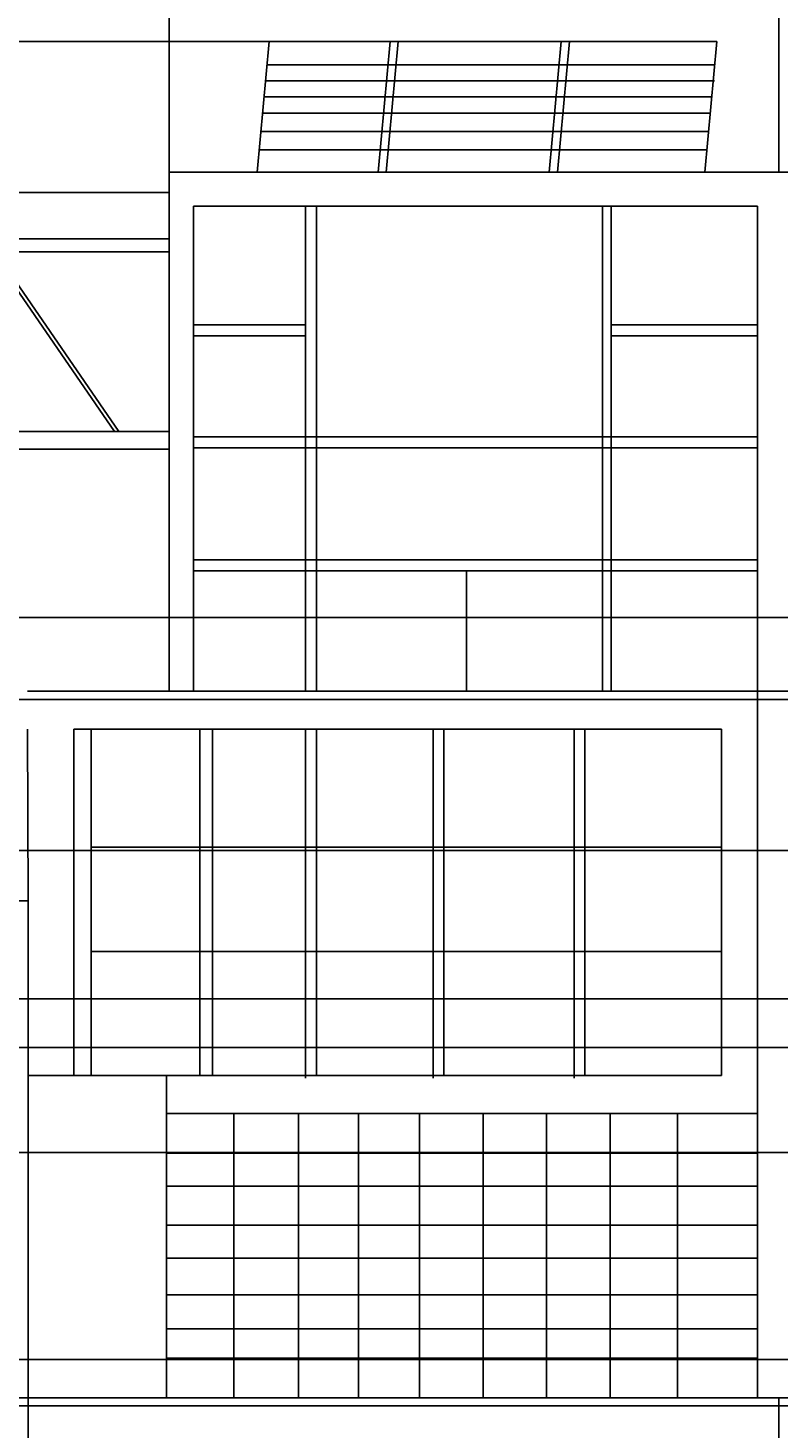
# Model space of a CAD drawing. Units: inches. Extents: x -32109 to 33221, y -19197 to 7608.
# Tile 5 of 25: x -6953 to -4279, y -16323 to -11338. Entities that reach past the tile are written whole.
import ezdxf

# ---------------------------------------------------------------- set-up
doc = ezdxf.new("R2010")
doc.units = ezdxf.units.IN
doc.header["$MEASUREMENT"] = 0
doc.layers.add('A-ANNO-DIMS', color=2, linetype='Continuous', lineweight=18)
doc.layers.add('A-ELEV', color=7, linetype='Continuous', lineweight=25)
doc.styles.get("Standard").update_dxf_attribs({"font": 'arial.ttf'})
doc.dimstyles.get("Standard").update_dxf_attribs({"dimtxt": 0.18, "dimasz": 0.18, "dimexe": 0.18, "dimexo": 0.0625, "dimgap": 0.09, "dimtad": 0, "dimtih": 1, "dimtoh": 1, "dimdec": 4, "dimzin": 0, "dimdsep": 46, "dimtxsty": 'Standard', "dimcen": 0.09, "dimadec": 0, "dimazin": 0, "dimtfac": 1, "dimtdec": 4, "dimtofl": 0, "dimtmove": 0, "dimatfit": 3, "dimfxl": 1, "dimtolj": 1, "dimtzin": 0, "dimarcsym": 0})

# ---------------------------------------------------------------- blocks, each defined once
blk = doc.blocks.new('*D13')
at = {"layer": 'A-ANNO-DIMS', "color": 0, "lineweight": -2, "transparency": 16777216}
for p, q in [((-21916.3, -16214.9), (-21916.3, -19197.3)), ((5067.2, -16244.2), (5067.2, -19197.3)), ((-21916.1, -19197.2), (-8425, -19197.2)), ((5067, -19197.2), (-8424.2, -19197.2))]:
    blk.add_line(p, q, dxfattribs=at)
at = {"layer": 'A-ANNO-DIMS', "color": 0, "transparency": 16777216}
for points in [[(-21916.1, -19197.1), (-21916.1, -19197.2), (-21916.3, -19197.2)], [(5067, -19197.1), (5067, -19197.2), (5067.2, -19197.2)]]:
    blk.add_solid(points, dxfattribs=at)
at = {"layer": 'Defpoints', "color": 0, "transparency": 16777216}
for p in [(-21916.3, -16214.8), (5067.2, -16244.1), (5067.2, -19197.2)]:
    blk.add_point(p, dxfattribs=at)
at = {"layer": 'A-ANNO-DIMS', "color": 0, "transparency": 16777216, "insert": (-8424.6, -19197.2), "char_height": 0.18, "attachment_point": 5}
blk.add_mtext('\\A1;26983', dxfattribs=at)
blk = doc.blocks.new('*D14')
at = {"layer": 'A-ANNO-DIMS', "color": 0, "lineweight": -2, "transparency": 16777216}
for p, q in [((-18893.9, -10978.7), (-32108.4, -10978.7)), ((-32108.2, -10978.9), (-32108.2, -13611.2)), ((-32108.2, -16243.9), (-32108.2, -13611.6)), ((5067.1, -16244.1), (-32108.4, -16244.1))]:
    blk.add_line(p, q, dxfattribs=at)
at = {"layer": 'A-ANNO-DIMS', "color": 0, "transparency": 16777216}
for points in [[(-32108.2, -10978.9), (-32108.2, -10978.9), (-32108.2, -10978.7)], [(-32108.2, -16243.9), (-32108.2, -16243.9), (-32108.2, -16244.1)]]:
    blk.add_solid(points, dxfattribs=at)
at = {"layer": 'Defpoints', "color": 0, "transparency": 16777216}
for p in [(-18893.8, -10978.7), (-32108.2, -16244.1), (5067.2, -16244.1)]:
    blk.add_point(p, dxfattribs=at)
at = {"layer": 'A-ANNO-DIMS', "color": 0, "transparency": 16777216, "insert": (-32108.2, -13611.4), "char_height": 0.18, "attachment_point": 5}
blk.add_mtext('\\A1;5265', dxfattribs=at)
blk = doc.blocks.new('*D15')
at = {"layer": 'A-ANNO-DIMS', "color": 0, "lineweight": -2, "transparency": 16777216}
for p, q in [((-8664.1, -16214.9), (-8664.1, -19197.3)), ((-6952.8, -16214.9), (-6952.8, -19197.3)), ((-8664, -19197.2), (-7808.9, -19197.2)), ((-6953, -19197.2), (-7808, -19197.2))]:
    blk.add_line(p, q, dxfattribs=at)
at = {"layer": 'A-ANNO-DIMS', "color": 0, "transparency": 16777216}
for points in [[(-8664, -19197.1), (-8664, -19197.2), (-8664.1, -19197.2)], [(-6953, -19197.1), (-6953, -19197.2), (-6952.8, -19197.2)]]:
    blk.add_solid(points, dxfattribs=at)
at = {"layer": 'Defpoints', "color": 0, "transparency": 16777216}
for p in [(-8664.1, -16214.8), (-6952.8, -16214.8), (-6952.8, -19197.2)]:
    blk.add_point(p, dxfattribs=at)
at = {"layer": 'A-ANNO-DIMS', "color": 0, "transparency": 16777216, "insert": (-7808.5, -19197.2), "char_height": 0.18, "attachment_point": 5}
blk.add_mtext('\\A1;1711.4', dxfattribs=at)
blk = doc.blocks.new('*D23')
at = {"layer": 'A-ANNO-DIMS', "color": 0, "lineweight": -2, "transparency": 16777216}
for p, q in [((-4093.7, -14968.1), (-32108.4, -14968.1)), ((-32108.2, -14968.3), (-32108.2, -15591.3)), ((-32108.2, -16214.6), (-32108.2, -15591.6)), ((-4279, -16214.8), (-32108.4, -16214.8))]:
    blk.add_line(p, q, dxfattribs=at)
at = {"layer": 'A-ANNO-DIMS', "color": 0, "transparency": 16777216}
for points in [[(-32108.2, -14968.3), (-32108.2, -14968.3), (-32108.2, -14968.1)], [(-32108.2, -16214.6), (-32108.2, -16214.6), (-32108.2, -16214.8)]]:
    blk.add_solid(points, dxfattribs=at)
at = {"layer": 'Defpoints', "color": 0, "transparency": 16777216}
for p in [(-32108.2, -14968.1), (-4093.7, -14968.1), (-4279, -16214.8)]:
    blk.add_point(p, dxfattribs=at)
at = {"layer": 'A-ANNO-DIMS', "color": 0, "transparency": 16777216, "insert": (-32108.2, -15591.4), "char_height": 0.18, "attachment_point": 5}
blk.add_mtext('\\A1;1246.7', dxfattribs=at)
blk = doc.blocks.new('*D88')
at = {"layer": 'A-ANNO-DIMS', "color": 0, "lineweight": -2, "transparency": 16777216}
for p, q in [((-6450, -11924), (-32108.4, -11924)), ((-32108.2, -11924.1), (-32108.2, -12380.7)), ((-32108.2, -12837.6), (-32108.2, -12381)), ((-6450, -12837.7), (-32108.4, -12837.7))]:
    blk.add_line(p, q, dxfattribs=at)
at = {"layer": 'A-ANNO-DIMS', "color": 0, "transparency": 16777216}
for points in [[(-32108.2, -11924.1), (-32108.2, -11924.1), (-32108.2, -11924)], [(-32108.2, -12837.6), (-32108.2, -12837.6), (-32108.2, -12837.7)]]:
    blk.add_solid(points, dxfattribs=at)
at = {"layer": 'Defpoints', "color": 0, "transparency": 16777216}
for p in [(-6450, -11924), (-32108.2, -12837.7), (-6450, -12837.7)]:
    blk.add_point(p, dxfattribs=at)
at = {"layer": 'A-ANNO-DIMS', "color": 0, "transparency": 16777216, "insert": (-32108.2, -12380.9), "char_height": 0.18, "attachment_point": 5}
blk.add_mtext('\\A1;913.8', dxfattribs=at)
blk = doc.blocks.new('*D92')
at = {"layer": 'A-ANNO-DIMS', "color": 0, "lineweight": -2, "transparency": 16777216}
for p, q in [((-8664.1, -13437.2), (9252.7, -13437.2)), ((9252.5, -13437.4), (9252.5, -14825.8)), ((9252.5, -16214.6), (9252.5, -14826.2)), ((-8664.1, -16214.8), (9252.7, -16214.8))]:
    blk.add_line(p, q, dxfattribs=at)
at = {"layer": 'A-ANNO-DIMS', "color": 0, "transparency": 16777216}
for points in [[(9252.5, -13437.4), (9252.5, -13437.4), (9252.5, -13437.2)], [(9252.5, -16214.6), (9252.5, -16214.6), (9252.5, -16214.8)]]:
    blk.add_solid(points, dxfattribs=at)
at = {"layer": 'Defpoints', "color": 0, "transparency": 16777216}
for p in [(-8664.1, -13437.2), (-8664.1, -16214.8), (9252.5, -16214.8)]:
    blk.add_point(p, dxfattribs=at)
at = {"layer": 'A-ANNO-DIMS', "color": 0, "transparency": 16777216, "insert": (9252.5, -14826), "char_height": 0.18, "attachment_point": 5}
blk.add_mtext('\\A1;2777.6', dxfattribs=at)
blk = doc.blocks.new('*D99')
at = {"layer": 'A-ANNO-DIMS', "color": 0, "lineweight": -2, "transparency": 16777216}
for p, q in [((-9175.1, -13729), (9252.7, -13729)), ((9252.5, -13729.2), (9252.5, -13997.5)), ((9252.5, -14266.2), (9252.5, -13997.9)), ((-9175.1, -14266.4), (9252.7, -14266.4))]:
    blk.add_line(p, q, dxfattribs=at)
at = {"layer": 'A-ANNO-DIMS', "color": 0, "transparency": 16777216}
for points in [[(9252.5, -13729.2), (9252.5, -13729.2), (9252.5, -13729)], [(9252.5, -14266.2), (9252.5, -14266.2), (9252.5, -14266.4)]]:
    blk.add_solid(points, dxfattribs=at)
at = {"layer": 'Defpoints', "color": 0, "transparency": 16777216}
for p in [(-9175.2, -13729), (-9175.2, -14266.4), (9252.5, -14266.4)]:
    blk.add_point(p, dxfattribs=at)
at = {"layer": 'A-ANNO-DIMS', "color": 0, "transparency": 16777216, "insert": (9252.5, -13997.7), "char_height": 0.18, "attachment_point": 5}
blk.add_mtext('\\A1;537.4', dxfattribs=at)
blk = doc.blocks.new('*D100')
at = {"layer": 'A-ANNO-DIMS', "color": 0, "lineweight": -2, "transparency": 16777216}
for p, q in [((-9175.1, -14266.4), (9252.7, -14266.4)), ((9252.5, -14266.6), (9252.5, -14530.6)), ((9252.5, -14794.9), (9252.5, -14530.9)), ((-9175.1, -14795.1), (9252.7, -14795.1))]:
    blk.add_line(p, q, dxfattribs=at)
at = {"layer": 'A-ANNO-DIMS', "color": 0, "transparency": 16777216}
for points in [[(9252.5, -14266.6), (9252.5, -14266.6), (9252.5, -14266.4)], [(9252.5, -14794.9), (9252.5, -14794.9), (9252.5, -14795.1)]]:
    blk.add_solid(points, dxfattribs=at)
at = {"layer": 'Defpoints', "color": 0, "transparency": 16777216}
for p in [(-9175.2, -14266.4), (-9175.2, -14795.1), (9252.5, -14795.1)]:
    blk.add_point(p, dxfattribs=at)
at = {"layer": 'A-ANNO-DIMS', "color": 0, "transparency": 16777216, "insert": (9252.5, -14530.7), "char_height": 0.18, "attachment_point": 5}
blk.add_mtext('\\A1;528.7', dxfattribs=at)
blk = doc.blocks.new('*D101')
at = {"layer": 'A-ANNO-DIMS', "color": 0, "lineweight": -2, "transparency": 16777216}
for p, q in [((-9175.1, -14795.1), (9252.7, -14795.1)), ((9252.5, -14795.3), (9252.5, -15068.4)), ((9252.5, -15341.8), (9252.5, -15068.7)), ((-9175.1, -15342), (9252.7, -15342))]:
    blk.add_line(p, q, dxfattribs=at)
at = {"layer": 'A-ANNO-DIMS', "color": 0, "transparency": 16777216}
for points in [[(9252.5, -14795.3), (9252.5, -14795.3), (9252.5, -14795.1)], [(9252.5, -15341.8), (9252.5, -15341.8), (9252.5, -15342)]]:
    blk.add_solid(points, dxfattribs=at)
at = {"layer": 'Defpoints', "color": 0, "transparency": 16777216}
for p in [(-9175.2, -14795.1), (-9175.2, -15342), (9252.5, -15342)]:
    blk.add_point(p, dxfattribs=at)
at = {"layer": 'A-ANNO-DIMS', "color": 0, "transparency": 16777216, "insert": (9252.5, -15068.6), "char_height": 0.18, "attachment_point": 5}
blk.add_mtext('\\A1;546.9', dxfattribs=at)
blk = doc.blocks.new('*D102')
at = {"layer": 'A-ANNO-DIMS', "color": 0, "lineweight": -2, "transparency": 16777216}
for p, q in [((-9175.1, -15342), (9252.7, -15342)), ((9252.5, -15342.2), (9252.5, -15710.5)), ((9252.5, -16079.1), (9252.5, -15710.8)), ((-9175.1, -16079.3), (9252.7, -16079.3))]:
    blk.add_line(p, q, dxfattribs=at)
at = {"layer": 'A-ANNO-DIMS', "color": 0, "transparency": 16777216}
for points in [[(9252.5, -15342.2), (9252.5, -15342.2), (9252.5, -15342)], [(9252.5, -16079.1), (9252.5, -16079.1), (9252.5, -16079.3)]]:
    blk.add_solid(points, dxfattribs=at)
at = {"layer": 'Defpoints', "color": 0, "transparency": 16777216}
for p in [(-9175.2, -15342), (-9175.2, -16079.3), (9252.5, -16079.3)]:
    blk.add_point(p, dxfattribs=at)
at = {"layer": 'A-ANNO-DIMS', "color": 0, "transparency": 16777216, "insert": (9252.5, -15710.6), "char_height": 0.18, "attachment_point": 5}
blk.add_mtext('\\A1;737.3', dxfattribs=at)
blk = doc.blocks.new('*D103')
at = {"layer": 'A-ANNO-DIMS', "color": 0, "lineweight": -2, "transparency": 16777216}
for p, q in [((-6952.8, -16214.9), (-6952.8, -19197.3)), ((-4279, -16214.9), (-4279, -19197.3)), ((-6952.6, -19197.2), (-5616.2, -19197.2)), ((-4279.1, -19197.2), (-5615.5, -19197.2))]:
    blk.add_line(p, q, dxfattribs=at)
at = {"layer": 'A-ANNO-DIMS', "color": 0, "transparency": 16777216}
for points in [[(-6952.6, -19197.1), (-6952.6, -19197.2), (-6952.8, -19197.2)], [(-4279.1, -19197.1), (-4279.1, -19197.2), (-4279, -19197.2)]]:
    blk.add_solid(points, dxfattribs=at)
at = {"layer": 'Defpoints', "color": 0, "transparency": 16777216}
for p in [(-6952.8, -16214.8), (-4279, -16214.8), (-4279, -19197.2)]:
    blk.add_point(p, dxfattribs=at)
at = {"layer": 'A-ANNO-DIMS', "color": 0, "transparency": 16777216, "insert": (-5615.9, -19197.2), "char_height": 0.18, "attachment_point": 5}
blk.add_mtext('\\A1;2674', dxfattribs=at)
blk = doc.blocks.new('*D104')
at = {"layer": 'A-ANNO-DIMS', "color": 0, "lineweight": -2, "transparency": 16777216}
for p, q in [((-4279, -16214.9), (-4279, -19197.3)), ((-2554.3, -16214.9), (-2554.3, -19197.3)), ((-4278.8, -19197.2), (-3417.1, -19197.2)), ((-2554.5, -19197.2), (-3416.2, -19197.2))]:
    blk.add_line(p, q, dxfattribs=at)
at = {"layer": 'A-ANNO-DIMS', "color": 0, "transparency": 16777216}
for points in [[(-4278.8, -19197.1), (-4278.8, -19197.2), (-4279, -19197.2)], [(-2554.5, -19197.1), (-2554.5, -19197.2), (-2554.3, -19197.2)]]:
    blk.add_solid(points, dxfattribs=at)
at = {"layer": 'Defpoints', "color": 0, "transparency": 16777216}
for p in [(-4279, -16214.8), (-2554.3, -16214.8), (-2554.3, -19197.2)]:
    blk.add_point(p, dxfattribs=at)
at = {"layer": 'A-ANNO-DIMS', "color": 0, "transparency": 16777216, "insert": (-3416.6, -19197.2), "char_height": 0.18, "attachment_point": 5}
blk.add_mtext('\\A1;1724.6', dxfattribs=at)
blk = doc.blocks.new('*D108')
at = {"layer": 'A-ANNO-DIMS', "color": 0, "lineweight": -2, "transparency": 16777216}
for p, q in [((-6450, -11850.7), (-6450, -7335)), ((-6449.8, -7335.2), (-5364.8, -7335.2)), ((-4279.1, -7335.2), (-5364.1, -7335.2)), ((-4279, -11850.7), (-4279, -7335))]:
    blk.add_line(p, q, dxfattribs=at)
at = {"layer": 'A-ANNO-DIMS', "color": 0, "transparency": 16777216}
for points in [[(-6449.8, -7335.1), (-6449.8, -7335.2), (-6450, -7335.2)], [(-4279.1, -7335.1), (-4279.1, -7335.2), (-4279, -7335.2)]]:
    blk.add_solid(points, dxfattribs=at)
at = {"layer": 'Defpoints', "color": 0, "transparency": 16777216}
for p in [(-4279, -7335.2), (-6450, -11850.8), (-4279, -11850.8)]:
    blk.add_point(p, dxfattribs=at)
at = {"layer": 'A-ANNO-DIMS', "color": 0, "transparency": 16777216, "insert": (-5364.5, -7335.2), "char_height": 0.18, "attachment_point": 5}
blk.add_mtext('\\A1;2171', dxfattribs=at)
blk = doc.blocks.new('*D110')
at = {"layer": 'A-ANNO-DIMS', "color": 0, "lineweight": -2, "transparency": 16777216}
for p, q in [((-6449.9, -11850.8), (9252.7, -11850.8)), ((9252.5, -11851), (9252.5, -14032.6)), ((9252.5, -16214.6), (9252.5, -14033)), ((-6952.7, -16214.8), (9252.7, -16214.8))]:
    blk.add_line(p, q, dxfattribs=at)
at = {"layer": 'A-ANNO-DIMS', "color": 0, "transparency": 16777216}
for points in [[(9252.5, -11851), (9252.5, -11851), (9252.5, -11850.8)], [(9252.5, -16214.6), (9252.5, -16214.6), (9252.5, -16214.8)]]:
    blk.add_solid(points, dxfattribs=at)
at = {"layer": 'Defpoints', "color": 0, "transparency": 16777216}
for p in [(-6450, -11850.8), (-6952.8, -16214.8), (9252.5, -16214.8)]:
    blk.add_point(p, dxfattribs=at)
at = {"layer": 'A-ANNO-DIMS', "color": 0, "transparency": 16777216, "insert": (9252.5, -14032.8), "char_height": 0.18, "attachment_point": 5}
blk.add_mtext('\\A1;4364', dxfattribs=at)
blk = doc.blocks.new('*D111')
at = {"layer": 'A-ANNO-DIMS', "color": 0, "lineweight": -2, "transparency": 16777216}
for p, q in [((-6954.6, -13699.5), (9252.7, -13699.5)), ((9252.5, -13699.6), (9252.5, -14957)), ((9252.5, -16214.6), (9252.5, -14957.3)), ((-6952.7, -16214.8), (9252.7, -16214.8))]:
    blk.add_line(p, q, dxfattribs=at)
at = {"layer": 'A-ANNO-DIMS', "color": 0, "transparency": 16777216}
for points in [[(9252.5, -13699.6), (9252.5, -13699.6), (9252.5, -13699.5)], [(9252.5, -16214.6), (9252.5, -16214.6), (9252.5, -16214.8)]]:
    blk.add_solid(points, dxfattribs=at)
at = {"layer": 'Defpoints', "color": 0, "transparency": 16777216}
for p in [(-6954.6, -13699.5), (-6952.8, -16214.8), (9252.5, -16214.8)]:
    blk.add_point(p, dxfattribs=at)
at = {"layer": 'A-ANNO-DIMS', "color": 0, "transparency": 16777216, "insert": (9252.5, -14957.1), "char_height": 0.18, "attachment_point": 5}
blk.add_mtext('\\A1;2515.4', dxfattribs=at)
blk = doc.blocks.new('*D159')
at = {"layer": 'A-ANNO-DIMS', "color": 0, "lineweight": -2, "transparency": 16777216}
for p, q in [((-6094.7, -11386.3), (-32108.4, -11386.3)), ((-32108.2, -11386.4), (-32108.2, -13800.4)), ((-32108.2, -16214.6), (-32108.2, -13800.7)), ((-6952.8, -16214.8), (-32108.4, -16214.8))]:
    blk.add_line(p, q, dxfattribs=at)
at = {"layer": 'A-ANNO-DIMS', "color": 0, "transparency": 16777216}
for points in [[(-32108.2, -11386.4), (-32108.2, -11386.4), (-32108.2, -11386.3)], [(-32108.2, -16214.6), (-32108.2, -16214.6), (-32108.2, -16214.8)]]:
    blk.add_solid(points, dxfattribs=at)
at = {"layer": 'Defpoints', "color": 0, "transparency": 16777216}
for p in [(-6094.7, -11386.3), (-32108.2, -16214.8), (-6952.8, -16214.8)]:
    blk.add_point(p, dxfattribs=at)
at = {"layer": 'A-ANNO-DIMS', "color": 0, "transparency": 16777216, "insert": (-32108.2, -13800.5), "char_height": 0.18, "attachment_point": 5}
blk.add_mtext('\\A1;4828.6', dxfattribs=at)

msp = doc.modelspace()

# ---------------------------------------------------------------- linework, layer by layer
at = {"layer": 'A-ELEV'}
for p, q in [((-6137.276, -11850.794), (-6094.672, -11386.256)), ((-4500.781, -11386.256), (-6094.672, -11386.256)), ((-5705.931, -11850.794), (-5663.327, -11386.256)), ((-5677.808, -11850.794), (-5635.204, -11386.256)), ((-5097.441, -11850.794), (-5054.836, -11386.256)), ((-5067.407, -11850.794), (-5024.803, -11386.256)), ((-5067.407, -11850.794), (-5024.803, -11386.256)), ((-4543.385, -11850.794), (-4500.781, -11386.256)), ((-4508.356, -11468.861), (-6102.248, -11468.861)), ((-4508.356, -11526.057), (-6107.493, -11526.057)), ((-4518.848, -11583.252), (-6112.739, -11583.252)), ((-4524.093, -11640.448), (-6117.984, -11640.448)), ((-4530.088, -11705.815), (-6123.979, -11705.815)), ((-4536.083, -11771.182), (-6129.974, -11771.182)), ((-4278.952, -11850.794), (-6449.955, -11850.794)), ((-6449.955, -11850.794), (-6449.955, -13699.459)), ((-6449.955, -11923.964), (-13434.383, -11923.964)), ((-4355.795, -11972.036), (-6363.956, -11972.036)), ((-6363.956, -11972.036), (-6363.956, -13699.459)), ((-4355.795, -11972.036), (-6363.956, -11972.036)), ((-5964.265, -11972.036), (-5964.265, -13699.459)), ((-5925.825, -11972.036), (-5925.825, -13699.459)), ((-4907.745, -11972.036), (-4907.745, -13699.459)), ((-4876.149, -11972.036), (-4876.149, -13699.459)), ((-4355.795, -13988.141), (-4355.795, -11972.036)), ((-13434.383, -12088.725), (-6449.955, -12088.725)), ((-6449.955, -12135.164), (-13434.383, -12135.164)), ((-6628.917, -12773.917), (-7071.065, -12132.707)), ((-6644.441, -12773.917), (-7068.778, -12158.535)), ((-5964.265, -12394.938), (-6363.956, -12394.938)), ((-4355.795, -12394.938), (-4876.149, -12394.938)), ((-5964.265, -12433.907), (-6363.956, -12433.907)), ((-4355.795, -12433.907), (-4876.149, -12433.907)), ((-13434.383, -12773.917), (-6449.955, -12773.917)), ((-4355.795, -12793.563), (-6363.956, -12793.563)), ((-6449.955, -12837.747), (-13434.383, -12837.747)), ((-4355.795, -12832.532), (-6363.956, -12832.532)), ((-4355.795, -13231.507), (-6363.956, -13231.507)), ((-4355.795, -13270.476), (-6363.956, -13270.476)), ((-5391.083, -13270.476), (-5391.083, -13699.459)), ((-5964.265, -13349.64), (-5964.265, -13699.459)), ((-6954.623, -13699.459), (-6943.296, -13699.459)), ((-6363.956, -13699.459), (-6943.296, -13699.459)), ((-5116.132, -13699.459), (-6363.956, -13699.459)), ((-5116.132, -13699.459), (-4355.795, -13699.459)), ((-6954.623, -13834.091), (-6952.774, -14445.256)), ((-6341.319, -13834.091), (-6789.778, -13834.091)), ((-6789.778, -13834.091), (-6789.778, -15067.104)), ((-6728.195, -15067.104), (-6728.195, -13834.091)), ((-6341.319, -15067.104), (-6341.319, -13834.091)), ((-6341.319, -13834.091), (-4483.388, -13834.091)), ((-6295.539, -15067.104), (-6295.539, -13834.091)), ((-5964.265, -13834.091), (-5964.265, -15077.062)), ((-5925.825, -13834.091), (-5925.825, -15067.104)), ((-5510.436, -13834.091), (-5510.436, -15077.062)), ((-5471.996, -13834.091), (-5471.996, -15067.104)), ((-5008.328, -13834.091), (-5008.328, -15077.062)), ((-4969.887, -13834.091), (-4969.887, -15067.104)), ((-4483.388, -13834.091), (-4483.388, -15067.104)), ((-4355.795, -13988.141), (-4355.795, -16214.811)), ((-6728.195, -14254.947), (-4483.388, -14254.947)), ((-6952.774, -14445.256), (-8891.72, -14445.256)), ((-6952.774, -14445.256), (-6952.774, -16214.811)), ((-6728.195, -14626.445), (-4483.388, -14626.445)), ((-6789.778, -15067.104), (-6952.774, -15067.104)), ((-6341.319, -15067.104), (-6789.778, -15067.104)), ((-6459.442, -15202.391), (-6459.442, -15067.104)), ((-6341.319, -15067.104), (-4483.388, -15067.104)), ((-6459.125, -15202.391), (-6459.442, -15202.391)), ((-6459.442, -16214.811), (-6459.442, -15202.391)), ((-6459.125, -15202.391), (-6341.319, -15202.391)), ((-6341.319, -15202.391), (-4483.388, -15202.391)), ((-6220.14, -16214.811), (-6220.14, -15202.391)), ((-5989.54, -16214.811), (-5989.54, -15202.391)), ((-5776.343, -16214.811), (-5776.343, -15202.391)), ((-5558.796, -16214.811), (-5558.796, -15202.391)), ((-5332.547, -16214.811), (-5332.547, -15202.391)), ((-5106.298, -16214.811), (-5106.298, -15202.391)), ((-4880.049, -16214.811), (-4880.049, -15202.391)), ((-4640.747, -16214.811), (-4640.747, -15202.391)), ((-4483.388, -15202.391), (-4355.795, -15202.391)), ((-6459.442, -15344.259), (-4355.795, -15344.259)), ((-6459.442, -15461.056), (-4355.795, -15461.056)), ((-6459.442, -15600.657), (-4355.795, -15600.657)), ((-6459.442, -15717.992), (-4355.795, -15717.992)), ((-6459.442, -15848.364), (-4355.795, -15848.364)), ((-6459.442, -15970.045), (-4355.795, -15970.045)), ((-6459.442, -16074.343), (-4355.795, -16074.343)), ((-12087.226, -16214.811), (7362.494, -16214.811)), ((-1417.009, -16214.811), (-10157.643, -16214.811)), ((-6952.774, -16214.811), (-4355.795, -16214.811)), ((-4278.952, -16214.811), (-4355.795, -16214.811))]:
    msp.add_line(p, q, dxfattribs=at)

# ---------------------------------------------------------------- dimensions: what is measured, and where the dimension line sits
at = {"layer": 'A-ANNO-DIMS'}
for base, p1, p2, override, picture, middle in [((-4278.952, -7335.16), (-6449.955, -11850.794), (-4278.952, -11850.794), {"dimdec": 0, "dimlfac": 1, "dimrnd": 0, "dimzin": 0, "dimdsep": 46, "dimlunit": 2}, '*D108', (-5364.454, -7335.16)), ((5067.151, -19197.169), (-21916.328, -16214.811), (5067.151, -16244.113), {"dimdec": 0, "dimlfac": 1, "dimrnd": 0, "dimzin": 0, "dimdsep": 46, "dimlunit": 2}, '*D13', (-8424.588, -19197.169)), ((-6952.774, -19197.169), (-8664.143, -16214.811), (-6952.774, -16214.811), {"dimdec": 1, "dimlfac": 1, "dimrnd": 0, "dimzin": 0, "dimdsep": 46, "dimlunit": 2}, '*D15', (-7808.458, -19197.169)), ((-4278.952, -19197.169), (-6952.774, -16214.811), (-4278.952, -16214.811), {"dimdec": 0, "dimlfac": 1, "dimrnd": 0, "dimzin": 0, "dimdsep": 46, "dimlunit": 2}, '*D103', (-5615.863, -19197.169)), ((-2554.321, -19197.169), (-4278.952, -16214.811), (-2554.321, -16214.811), {"dimdec": 1, "dimlfac": 1, "dimrnd": 0, "dimzin": 0, "dimdsep": 46, "dimlunit": 2}, '*D104', (-3416.636, -19197.169))]:
    dim = msp.add_linear_dim(base=base, p1=p1, p2=p2, dimstyle='Standard', override=override, dxfattribs=at)
    dim.commit()
    dim.dimension.update_dxf_attribs({"geometry": picture, "text_midpoint": middle})
for base, p1, p2, override, picture, middle in [((-32108.187, -16244.113), (-18893.845, -10978.73), (5067.151, -16244.113), {"dimdec": 0, "dimlfac": 1, "dimrnd": 0, "dimzin": 0, "dimdsep": 46, "dimlunit": 2}, '*D14', (-32108.187, -13611.422)), ((-32108.187, -16214.811), (-6094.672, -11386.256), (-6952.774, -16214.811), {"dimdec": 1, "dimlfac": 1, "dimrnd": 0, "dimzin": 0, "dimdsep": 46, "dimlunit": 2}, '*D159', (-32108.187, -13800.533)), ((9252.494, -16214.811), (-6449.955, -11850.794), (-6952.774, -16214.811), {"dimdec": 0, "dimlfac": 1, "dimrnd": 0, "dimzin": 0, "dimdsep": 46, "dimlunit": 2}, '*D110', (9252.494, -14032.802)), ((-32108.187, -12837.747), (-6449.955, -11923.964), (-6449.955, -12837.747), {"dimdec": 1, "dimlfac": 1, "dimrnd": 0, "dimzin": 0, "dimdsep": 46, "dimlunit": 2}, '*D88', (-32108.187, -12380.856)), ((9252.494, -16214.811), (-8664.143, -13437.203), (-8664.143, -16214.811), {"dimdec": 1, "dimlfac": 1, "dimrnd": 0, "dimzin": 0, "dimdsep": 46, "dimlunit": 2}, '*D92', (9252.494, -14826.007)), ((9252.494, -16214.811), (-6954.623, -13699.459), (-6952.774, -16214.811), {"dimdec": 1, "dimlfac": 1, "dimrnd": 0, "dimzin": 0, "dimdsep": 46, "dimlunit": 2}, '*D111', (9252.494, -14957.135)), ((9252.494, -14266.38), (-9175.157, -13729.028), (-9175.157, -14266.38), {"dimdec": 1, "dimlfac": 1, "dimrnd": 0, "dimzin": 0, "dimdsep": 46, "dimlunit": 2}, '*D99', (9252.494, -13997.704)), ((9252.494, -14795.117), (-9175.157, -14266.38), (-9175.157, -14795.117), {"dimdec": 1, "dimlfac": 1, "dimrnd": 0, "dimzin": 0, "dimdsep": 46, "dimlunit": 2}, '*D100', (9252.494, -14530.748)), ((9252.494, -15341.992), (-9175.157, -14795.117), (-9175.157, -15341.992), {"dimdec": 1, "dimlfac": 1, "dimrnd": 0, "dimzin": 0, "dimdsep": 46, "dimlunit": 2}, '*D101', (9252.494, -15068.555)), ((-32108.187, -14968.079), (-4278.952, -16214.811), (-4093.675, -14968.079), {"dimdec": 1, "dimlfac": 1, "dimrnd": 0, "dimzin": 0, "dimdsep": 46, "dimlunit": 2}, '*D23', (-32108.187, -15591.445)), ((9252.494, -16079.3), (-9175.157, -15341.992), (-9175.157, -16079.3), {"dimdec": 1, "dimlfac": 1, "dimrnd": 0, "dimzin": 0, "dimdsep": 46, "dimlunit": 2}, '*D102', (9252.494, -15710.646))]:
    dim = msp.add_linear_dim(base=base, p1=p1, p2=p2, angle=90, dimstyle='Standard', override=override, dxfattribs=at)
    dim.commit()
    dim.dimension.update_dxf_attribs({"geometry": picture, "text_midpoint": middle})

doc.saveas('drawing.dxf')
